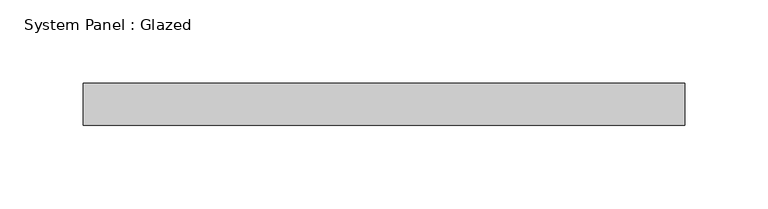
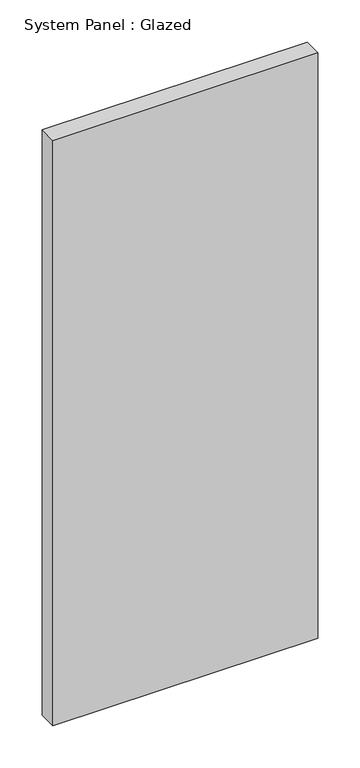
"""IFC4 building model written with IfcOpenShell, lengths in millimetres: plate geometry, System Panel : Glazed."""

from ifc_helpers import new_model, si_unit, origin, origin_with_axes, place, context, project, spatial, polyline, outline, extrude, source, transform, mapped, element, save


def system_panel_glazed_f45b48ac(model_context):
    return source(origin(), model_context, "Body", "SweptSolid", [
        extrude(outline(polyline([(180.975, 19.05), (-180.975, 19.05), (-180.975, 44.45), (180.975, 44.45), (180.975, 19.05)])), origin_with_axes(), (0.0, 0.0, 1.0), 845.6662788),
    ])


if __name__ == "__main__":
    model = new_model("IFC4")
    model_context = context("Model", 3, world=origin())
    ifc_project = project(units=[si_unit("LENGTHUNIT", "METRE", prefix="MILLI")], contexts=[model_context])
    site = spatial("IfcSite", under=ifc_project)
    building = spatial("IfcBuilding", under=site)
    placement = place(None, origin())
    system_panel_glazed_shape = system_panel_glazed_f45b48ac(model_context)
    element("IfcPlate", 1, ObjectType="System Panel : Glazed", at=placement, inside=building, context=model_context, shape_type="MappedRepresentation", body=[
        mapped(system_panel_glazed_shape, transform((0.0, 0.0, 0.0), x_axis=(1.0, 0.0, 0.0), y_axis=(0.0, 1.0, 0.0), z_axis=(0.0, 0.0, 1.0))),
    ])
    save(model, "model.ifc")

# Revit data of these elements
# Type "System Panel : Glazed"
#   Construction Type Id = "GSP4R"
#   Analytic Construction = "1/8 in Pilkington single glazing"
#   Visual Light Transmittance = 0.9
#   Solar Heat Gain Coefficient = 0.86
#   Heat Transfer Coefficient (U) = 1.18115 BTU/(h·ft²·°F)
#   Define Thermal Properties by = 1
# Element 1 (IfcPlate, "System Panel : Glazed")
#   Materials on its faces: "Glass"
# Materials
#   "Glass": class "Glass", colour RGB 0 128 192, transparency 0.75, Description = "Soda Lime Glass", Cost = 0
